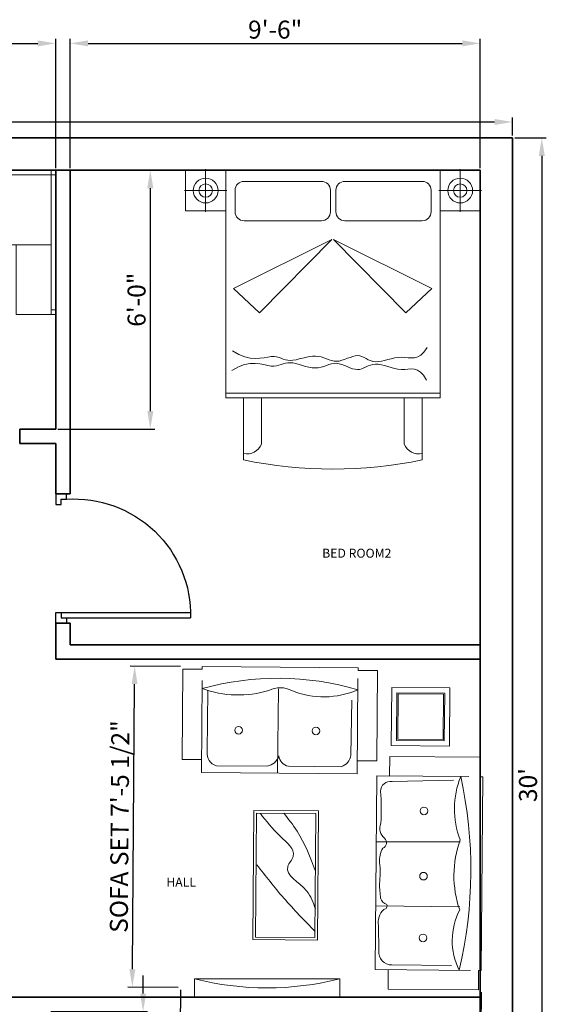
# Model space of a CAD drawing. Units: inches. Extents: x -24887 to 3061, y 1794 to 4919553.
# Tile 7 of 14: x 2328 to 2474, y 2076 to 2350. Entities that reach past the tile are written whole.
import ezdxf

# ---------------------------------------------------------------- set-up
doc = ezdxf.new("R2010")
doc.units = ezdxf.units.IN
for name, color, linetype, lineweight in [('A-ANNO-DIMS', 2, 'Continuous', 18), ('A-AREA-IDEN', 7, 'Continuous', 18), ('A-FURN', 8, 'Continuous', 18), ('door', 4, 'Continuous', 25), ('TV', 210, 'Continuous', 18), ('wall', 7, 'Continuous', 35)]:
    doc.layers.add(name, color=color, linetype=linetype, lineweight=lineweight)
doc.styles.get("Standard").update_dxf_attribs({"font": 'arial.ttf'})
doc.dimstyles.new('ISO-25', dxfattribs={"dimtxt": 5, "dimasz": 5, "dimexe": 1.25, "dimexo": 0.625, "dimtad": 1, "dimdec": 1, "dimlunit": 3, "dimtxsty": 'Standard', "dimcen": 2.5, "dimadec": 0, "dimazin": 0, "dimtfac": 1, "dimtdec": 1, "dimtmove": 0, "dimatfit": 3, "dimfxl": 1, "dimarcsym": 0})

# ---------------------------------------------------------------- blocks, each defined once
blk = doc.blocks.new('A$C4F543DC7')
for p, q in [((0.013, 3.35, -0.169), (3.313, 3.35, -0.169)), ((0.463, 3.35, -0.169), (0.013, 3.35, -0.169)), ((0.013, 2.896, -0.169), (0.013, 3.35, -0.169)), ((0.013, 3.35, -0.169), (0.013, 2.896, -0.169)), ((0.238, 3.123, -0.439), (0.238, 3.361, -0.439)), ((0.463, 3.35, -0.169), (0.463, 0.8, -0.169)), ((2.863, 3.35, -0.169), (0.463, 3.35, -0.169)), ((0.463, 2.896, -0.169), (0.463, 3.35, -0.169)), ((2.863, 0.8, -0.169), (2.863, 3.35, -0.169)), ((2.863, 3.35, -0.169), (3.313, 3.35, -0.169)), ((2.863, 2.896, -0.169), (2.863, 3.35, -0.169)), ((3.089, 3.123, -0.439), (3.089, 3.361, -0.439)), ((3.313, 3.35, -0.169), (3.313, 2.896, -0.169)), ((3.313, 3.35, -0.169), (3.313, 2.896, -0.169)), ((1.535, 3.226, -0.169), (0.668, 3.226, -0.169)), ((2.664, 3.226, -0.169), (1.797, 3.226, -0.169)), ((0.238, 3.123, -0.439), (0, 3.123, -0.439)), ((0.238, 3.123, -0.439), (0.476, 3.123, -0.439)), ((0.238, 3.123, -0.439), (0.238, 2.885, -0.439)), ((0.568, 3.126, -0.169), (0.568, 2.884, -0.169)), ((1.635, 2.884, -0.169), (1.635, 3.126, -0.169)), ((1.697, 3.126, -0.169), (1.697, 2.884, -0.169)), ((2.764, 2.884, -0.169), (2.764, 3.126, -0.169)), ((3.089, 3.123, -0.439), (2.851, 3.123, -0.439)), ((3.089, 3.123, -0.439), (3.089, 2.885, -0.439)), ((3.089, 3.123, -0.439), (3.327, 3.123, -0.439)), ((0.463, 2.896, -0.169), (0.013, 2.896, -0.169)), ((0.013, 2.896, -0.169), (0.463, 2.896, -0.169)), ((0.463, 0.8, -0.169), (0.463, 2.896, -0.169)), ((2.863, 2.896, -0.169), (2.863, 0.8, -0.169)), ((3.313, 2.896, -0.169), (2.863, 2.896, -0.169)), ((3.313, 2.896, -0.169), (2.863, 2.896, -0.169)), ((0.668, 2.784, -0.169), (1.535, 2.784, -0.169)), ((1.797, 2.784, -0.169), (2.664, 2.784, -0.169)), ((1.653, 2.573, -0.169), (0.55, 2.025, -0.169)), ((0.841, 1.752, -0.169), (1.653, 2.573, -0.169)), ((2.481, 1.752, -0.169), (1.669, 2.573, -0.169)), ((1.669, 2.573, -0.169), (2.772, 2.025, -0.169)), ((0.55, 2.025, -0.169), (0.841, 1.752, -0.169)), ((2.772, 2.025, -0.169), (2.481, 1.752, -0.169)), ((0.537, 1.327, -0.169), (0.609, 1.284, -0.169)), ((2.683, 1.312, -0.169), (2.718, 1.364, -0.169)), ((0.609, 1.284, -0.169), (0.676, 1.257, -0.169)), ((0.676, 1.257, -0.169), (0.737, 1.243, -0.169)), ((0.737, 1.243, -0.169), (0.794, 1.239, -0.169)), ((0.794, 1.239, -0.169), (0.846, 1.242, -0.169)), ((0.846, 1.242, -0.169), (0.893, 1.249, -0.169)), ((0.893, 1.249, -0.169), (0.935, 1.256, -0.169)), ((0.935, 1.256, -0.169), (0.972, 1.261, -0.169)), ((0.972, 1.261, -0.169), (1.004, 1.262, -0.169)), ((1.004, 1.262, -0.169), (1.033, 1.258, -0.169)), ((1.033, 1.258, -0.169), (1.06, 1.251, -0.169)), ((1.06, 1.251, -0.169), (1.084, 1.242, -0.169)), ((1.084, 1.242, -0.169), (1.108, 1.234, -0.169)), ((1.108, 1.234, -0.169), (1.132, 1.226, -0.169)), ((1.132, 1.226, -0.169), (1.158, 1.22, -0.169)), ((1.158, 1.22, -0.169), (1.185, 1.218, -0.169)), ((1.185, 1.218, -0.169), (1.216, 1.22, -0.169)), ((1.216, 1.22, -0.169), (1.25, 1.226, -0.169)), ((1.25, 1.226, -0.169), (1.285, 1.235, -0.169)), ((1.285, 1.235, -0.169), (1.322, 1.244, -0.169)), ((1.322, 1.244, -0.169), (1.359, 1.253, -0.169)), ((1.359, 1.253, -0.169), (1.396, 1.261, -0.169)), ((1.396, 1.261, -0.169), (1.433, 1.266, -0.169)), ((1.433, 1.266, -0.169), (1.468, 1.268, -0.169)), ((1.468, 1.268, -0.169), (1.501, 1.264, -0.169)), ((1.501, 1.264, -0.169), (1.532, 1.257, -0.169)), ((1.532, 1.257, -0.169), (1.562, 1.247, -0.169)), ((1.562, 1.247, -0.169), (1.591, 1.237, -0.169)), ((1.591, 1.237, -0.169), (1.62, 1.226, -0.169)), ((1.62, 1.226, -0.169), (1.648, 1.217, -0.169)), ((1.648, 1.217, -0.169), (1.676, 1.211, -0.169)), ((1.735, 1.212, -0.169), (1.765, 1.22, -0.169)), ((1.765, 1.22, -0.169), (1.795, 1.23, -0.169)), ((1.795, 1.23, -0.169), (1.826, 1.242, -0.169)), ((1.826, 1.242, -0.169), (1.856, 1.253, -0.169)), ((1.856, 1.253, -0.169), (1.885, 1.263, -0.169)), ((1.885, 1.263, -0.169), (1.913, 1.27, -0.169)), ((1.913, 1.27, -0.169), (1.94, 1.272, -0.169)), ((1.94, 1.272, -0.169), (1.965, 1.269, -0.169)), ((1.965, 1.269, -0.169), (1.989, 1.262, -0.169)), ((1.989, 1.262, -0.169), (2.012, 1.251, -0.169)), ((2.012, 1.251, -0.169), (2.036, 1.239, -0.169)), ((2.036, 1.239, -0.169), (2.06, 1.227, -0.169)), ((2.06, 1.227, -0.169), (2.085, 1.216, -0.169)), ((2.085, 1.216, -0.169), (2.112, 1.208, -0.169)), ((2.206, 1.21, -0.169), (2.242, 1.218, -0.169)), ((2.242, 1.218, -0.169), (2.279, 1.228, -0.169)), ((2.279, 1.228, -0.169), (2.317, 1.238, -0.169)), ((2.317, 1.238, -0.169), (2.356, 1.246, -0.169)), ((2.356, 1.246, -0.169), (2.394, 1.253, -0.169)), ((2.394, 1.253, -0.169), (2.433, 1.255, -0.169)), ((2.433, 1.255, -0.169), (2.47, 1.253, -0.169)), ((2.47, 1.253, -0.169), (2.506, 1.249, -0.169)), ((2.506, 1.249, -0.169), (2.542, 1.246, -0.169)), ((2.542, 1.246, -0.169), (2.578, 1.248, -0.169)), ((2.578, 1.248, -0.169), (2.613, 1.257, -0.169)), ((2.613, 1.257, -0.169), (2.648, 1.277, -0.169)), ((2.648, 1.277, -0.169), (2.683, 1.312, -0.169)), ((0.533, 1.105, -0.169), (0.607, 1.146, -0.169)), ((0.607, 1.146, -0.169), (0.674, 1.171, -0.169)), ((0.674, 1.171, -0.169), (0.736, 1.183, -0.169)), ((0.736, 1.183, -0.169), (0.793, 1.185, -0.169)), ((0.793, 1.185, -0.169), (0.845, 1.18, -0.169)), ((0.845, 1.18, -0.169), (0.891, 1.172, -0.169)), ((0.891, 1.172, -0.169), (0.933, 1.163, -0.169)), ((0.933, 1.163, -0.169), (0.97, 1.156, -0.169)), ((0.97, 1.156, -0.169), (1.003, 1.155, -0.169)), ((1.003, 1.155, -0.169), (1.032, 1.158, -0.169)), ((1.032, 1.158, -0.169), (1.058, 1.164, -0.169)), ((1.058, 1.164, -0.169), (1.083, 1.172, -0.169)), ((1.083, 1.172, -0.169), (1.107, 1.18, -0.169)), ((1.107, 1.18, -0.169), (1.132, 1.187, -0.169)), ((1.132, 1.187, -0.169), (1.157, 1.192, -0.169)), ((1.157, 1.192, -0.169), (1.185, 1.193, -0.169)), ((1.185, 1.193, -0.169), (1.216, 1.19, -0.169)), ((1.216, 1.19, -0.169), (1.249, 1.183, -0.169)), ((1.249, 1.183, -0.169), (1.284, 1.173, -0.169)), ((1.284, 1.173, -0.169), (1.321, 1.163, -0.169)), ((1.321, 1.163, -0.169), (1.358, 1.152, -0.169)), ((1.358, 1.152, -0.169), (1.394, 1.143, -0.169)), ((1.394, 1.143, -0.169), (1.431, 1.137, -0.169)), ((1.431, 1.137, -0.169), (1.466, 1.135, -0.169)), ((1.466, 1.135, -0.169), (1.499, 1.137, -0.169)), ((1.499, 1.137, -0.169), (1.531, 1.143, -0.169)), ((1.531, 1.143, -0.169), (1.561, 1.152, -0.169)), ((1.561, 1.152, -0.169), (1.59, 1.162, -0.169)), ((1.59, 1.162, -0.169), (1.619, 1.172, -0.169)), ((1.619, 1.172, -0.169), (1.648, 1.18, -0.169)), ((1.648, 1.18, -0.169), (1.676, 1.185, -0.169)), ((1.676, 1.211, -0.169), (1.705, 1.209, -0.169)), ((1.676, 1.185, -0.169), (1.705, 1.186, -0.169)), ((1.705, 1.209, -0.169), (1.735, 1.212, -0.169)), ((1.705, 1.186, -0.169), (1.734, 1.182, -0.169)), ((1.734, 1.182, -0.169), (1.764, 1.173, -0.169)), ((1.764, 1.173, -0.169), (1.794, 1.162, -0.169)), ((1.794, 1.162, -0.169), (1.824, 1.149, -0.169)), ((1.824, 1.149, -0.169), (1.854, 1.137, -0.169)), ((1.854, 1.137, -0.169), (1.883, 1.126, -0.169)), ((1.883, 1.126, -0.169), (1.911, 1.119, -0.169)), ((1.911, 1.119, -0.169), (1.937, 1.115, -0.169)), ((1.937, 1.115, -0.169), (1.963, 1.118, -0.169)), ((1.963, 1.118, -0.169), (1.987, 1.124, -0.169)), ((1.987, 1.124, -0.169), (2.011, 1.134, -0.169)), ((2.011, 1.134, -0.169), (2.034, 1.145, -0.169)), ((2.034, 1.145, -0.169), (2.059, 1.157, -0.169)), ((2.059, 1.157, -0.169), (2.084, 1.167, -0.169)), ((2.084, 1.167, -0.169), (2.111, 1.174, -0.169)), ((2.111, 1.174, -0.169), (2.14, 1.177, -0.169)), ((2.112, 1.208, -0.169), (2.141, 1.204, -0.169)), ((2.14, 1.177, -0.169), (2.172, 1.175, -0.169)), ((2.141, 1.204, -0.169), (2.172, 1.205, -0.169)), ((2.172, 1.205, -0.169), (2.206, 1.21, -0.169)), ((2.172, 1.175, -0.169), (2.206, 1.169, -0.169)), ((2.206, 1.169, -0.169), (2.241, 1.16, -0.169)), ((2.241, 1.16, -0.169), (2.278, 1.149, -0.169)), ((2.278, 1.149, -0.169), (2.316, 1.138, -0.169)), ((2.316, 1.138, -0.169), (2.354, 1.128, -0.169)), ((2.354, 1.128, -0.169), (2.392, 1.121, -0.169)), ((2.392, 1.121, -0.169), (2.43, 1.117, -0.169)), ((2.43, 1.117, -0.169), (2.468, 1.118, -0.169)), ((2.468, 1.118, -0.169), (2.504, 1.121, -0.169)), ((2.504, 1.121, -0.169), (2.54, 1.123, -0.169)), ((2.54, 1.123, -0.169), (2.576, 1.12, -0.169)), ((2.576, 1.12, -0.169), (2.611, 1.109, -0.169)), ((2.611, 1.109, -0.169), (2.645, 1.088, -0.169)), ((2.645, 1.088, -0.169), (2.679, 1.052, -0.169)), ((2.679, 1.052, -0.169), (2.712, 0.999, -0.169)), ((0.463, 0.85, -0.169), (2.863, 0.85, -0.169)), ((0.463, 0.8, -0.169), (2.863, 0.8, -0.169)), ((0.663, 0.8, -0.169), (0.463, 0.8, -0.169)), ((0.663, 0.8, -0.169), (2.663, 0.8, -0.169)), ((0.663, 0.104, -0.169), (0.663, 0.8, -0.169)), ((0.663, 0.104, -0.169), (0.663, 0.8, -0.169)), ((0.863, 0.281, -0.169), (0.863, 0.8, -0.169)), ((2.463, 0.8, -0.169), (2.463, 0.281, -0.169)), ((2.863, 0.8, -0.169), (2.663, 0.8, -0.169)), ((2.663, 0.8, -0.169), (2.663, 0.104, -0.169)), ((2.663, 0.8, -0.169), (2.663, 0.104, -0.169))]:
    blk.add_line(p, q)
for centre, radius in [((0.238, 3.123, -0.439), 0.139), ((3.089, 3.123, -0.439), 0.139), ((0.238, 3.123, -0.439), 0.075), ((3.089, 3.123, -0.439), 0.075)]:
    blk.add_circle(centre, radius)
for centre, radius, start, end in [((0.668, 3.126, -0.169), 0.1, 90, 180), ((1.535, 3.126, -0.169), 0.1, 0, 90), ((1.797, 3.126, -0.169), 0.1, 90, 180), ((2.664, 3.126, -0.169), 0.1, 0, 90), ((0.668, 2.884, -0.169), 0.1, 180, 270), ((1.535, 2.884, -0.169), 0.1, 270, 0), ((1.797, 2.884, -0.169), 0.1, 180, 270), ((2.664, 2.884, -0.169), 0.1, 270, 0), ((0.699, 0.347, -0.169), 0.177, 258.2616, 338.032), ((2.627, 0.347, -0.169), 0.177, 201.968, 281.7384), ((1.663, 4.86, -0.169), 4.86, 258.1252, 281.8748), ((1.663, 4.86, -0.169), 4.86, 258.1252, 281.8748)]:
    blk.add_arc(centre, radius, start, end)
blk = doc.blocks.new('A$C412119AE')
for p, q in [((1765.9, 2176), (1765.9, 2326)), ((1765.9, 2326), (2465.9, 2326)), ((2465.9, 2326), (2465.9, 2176)), ((1665.9, 2176), (1765.9, 2176)), ((1665.9, 2176), (1665.9, 970.8)), ((2379.1, 2176), (1665.9, 2176)), ((2465.9, 2176), (2485.9, 2176)), ((2485.9, 2176), (2485.9, 970.8)), ((1719.4, 1668.1), (1719.4, 2061.3)), ((1825.7, 2132.2), (2302.7, 2132.2)), ((1375.4, 1768.9), (375.4, 1768.9)), ((375.4, 1768.9), (375.4, 1268.9)), ((1375.4, 1268.9), (1375.4, 1768.9)), ((1355.4, 1748.9), (395.4, 1748.9)), ((395.4, 1748.9), (395.4, 1288.9)), ((1355.4, 1288.9), (1355.4, 1748.9)), ((1669.2, 1587.6), (2319.2, 1585.7)), ((1719.4, 1094.5), (1719.4, 1503.8)), ((375.4, 1268.9), (1375.4, 1268.9)), ((395.4, 1288.9), (1355.4, 1288.9)), ((2235, 1017.2), (1809.6, 1020.4)), ((1665.9, 970.8), (2404.3, 970.8)), ((1765.9, 820.8), (1765.9, 970.8)), ((2485.9, 970.8), (2465.9, 970.8)), ((2465.9, 970.8), (2465.9, 820.8)), ((150, 820), (150, 81.6)), ((1650, 820), (150, 820)), ((490.8, 797.2), (296.7, 793)), ((642.7, 820), (640.8, 170)), ((1139.6, 820), (1143.5, 170)), ((1650, 106.9), (1650, 820)), ((1650, 820), (1650, 720)), ((2465.9, 820.8), (1765.9, 820.8)), ((0, 20), (0, 720)), ((0, 720), (150, 720)), ((187.2, 692), (187.2, 228.9)), ((1620.5, 224.7), (1607.9, 700.4)), ((1650, 720), (1800, 720)), ((1800, 720), (1800, 20)), ((1885.8, 708.9), (1885.8, 258.9)), ((2335.8, 708.9), (1885.8, 708.9)), ((2335.8, 258.9), (2335.8, 708.9)), ((1925.8, 668.9), (1925.8, 298.9)), ((2295.8, 668.9), (1925.8, 668.9)), ((1935.8, 658.9), (1935.8, 308.9)), ((2285.8, 658.9), (1935.8, 658.9)), ((2285.8, 308.9), (2285.8, 658.9)), ((2295.8, 298.9), (2295.8, 668.9)), ((1935.8, 308.9), (2285.8, 308.9)), ((1885.8, 258.9), (2335.8, 258.9)), ((1925.8, 298.9), (2295.8, 298.9)), ((150, 20), (0, 20)), ((150, 0), (150, 20)), ((1650, 20), (1650, 0)), ((1800, 20), (1650, 20)), ((1650, 0), (150, 0))]:
    blk.add_line(p, q)
for centre in [(1995.2, 1891.7), (1995.2, 1293.1), (398.2, 452), (876.5, 452), (1381.8, 452)]:
    blk.add_circle(centre, 29.5)
for centre, radius, start, end in [((3089.3, 1902.2), 820.4, 160.50304, 197.27883), ((202.9, 1573.4), 2197.3, 344.08302, 15.91698), ((1812.8, 2036.4), 96.7, 82.30019, 165.08006), ((1830, 1685.8), 112, 189.0797, 254.44081), ((2133.5, 1569.9), 193.8, 332.79347, 27.20653), ((1809.1, 1487.1), 91.2, 95.74421, 169.48399), ((2917.4, 1237.9), 658.1, 158.30056, 203.94833), ((1824.2, 1130.1), 110.7, 198.77187, 262.42669), ((284.9, 696), 97.7, 83.05444, 182.36446), ((516, 656.3), 143.2, 45.31905, 100.10139), ((721.1, 716.6), 67.9, 104.67166, 165.32844), ((1108.9, -2844), 3648.9, 94.62092, 96.37281), ((897.6, 1374.7), 587.5, 261.9179, 278.0821), ((996.1, 612.3), 181.4, 58.97104, 95.03964), ((1133, 788.8), 48.2, 205.88938, 315.66926), ((1244.1, 695.8), 96.9, 66.28266, 142.29634), ((1373.1, 2811.3), 2028.7, 267.45837, 274.48249), ((1532.5, 712.5), 76.3, 350.88786, 90.69758), ((643.8, 758.5), 27.2, 180.80594, 295.18319), ((383.4, -290.5), 516.3, 63.11882, 116.88118), ((900, 3466.4), 3380.7, 257.18237, 282.81763), ((888.2, -595.2), 811.8, 70.47891, 109.52109), ((1404.7, -453), 669.5, 68.50957, 111.49043)]:
    blk.add_arc(centre, radius, start, end)
for points, knots in [([(954.7, 1741.3), (867.9, 1672.9), (688.2, 1531.3), (525.8, 1370), (441.9, 1286.7)], [0, 0, 0, 0, 331.319965, 685.817203, 685.817203, 685.817203, 685.817203]), ([(1351, 1718), (1294.3, 1672.1), (1194, 1591.1), (1053.5, 1416.2), (895.9, 1563.2), (786.6, 1342.9), (665.1, 1302.7), (616.7, 1286.7)], [0, 0, 0, 0, 235.219039, 416.259432, 507.480442, 744.13898, 900.517858, 900.517858, 900.517858, 900.517858]), ([(1356.8, 1537.3), (1311.3, 1500.6), (1176.6, 1392.3), (1015, 1328.7), (908.1, 1286.7)], [0, 0, 0, 0, 174.836893, 516.353531, 516.353531, 516.353531, 516.353531])]:
    blk.add_open_spline(points, degree=3, knots=knots)
blk = doc.blocks.new('*D30')
at = {"layer": 'A-ANNO-DIMS', "color": 0, "lineweight": -2, "transparency": 16777216}
for p, q in [((2164.92, 2317.57), (2164.92, 2322.63)), ((2464.92, 2317.57), (2464.92, 2322.63)), ((2169.92, 2321.38), (2459.92, 2321.38))]:
    blk.add_line(p, q, dxfattribs=at)
at = {"layer": 'A-ANNO-DIMS', "color": 0, "transparency": 16777216}
for points in [[(2169.92, 2322.21), (2169.92, 2320.55), (2164.92, 2321.38)], [(2459.92, 2322.21), (2459.92, 2320.55), (2464.92, 2321.38)]]:
    blk.add_solid(points, dxfattribs=at)
at = {"layer": 'Defpoints', "color": 0, "transparency": 16777216}
for p in [(2464.92, 2321.38), (2164.92, 2316.94), (2464.92, 2316.94)]:
    blk.add_point(p, dxfattribs=at)
at = {"layer": 'A-ANNO-DIMS', "color": 0, "transparency": 16777216, "insert": (2314.92, 2324.56), "char_height": 5, "attachment_point": 5}
blk.add_mtext("25'", dxfattribs=at)
blk = doc.blocks.new('*D31')
at = {"layer": 'A-ANNO-DIMS', "color": 0, "lineweight": -2, "transparency": 16777216}
for p, q in [((2465.55, 2316.94), (2474.28, 2316.94)), ((2473.03, 2311.94), (2473.03, 1961.94)), ((2465.55, 1956.94), (2474.28, 1956.94))]:
    blk.add_line(p, q, dxfattribs=at)
at = {"layer": 'A-ANNO-DIMS', "color": 0, "transparency": 16777216}
for points in [[(2472.2, 2311.94), (2473.87, 2311.94), (2473.03, 2316.94)], [(2472.2, 1961.94), (2473.87, 1961.94), (2473.03, 1956.94)]]:
    blk.add_solid(points, dxfattribs=at)
at = {"layer": 'Defpoints', "color": 0, "transparency": 16777216}
for p in [(2464.92, 2316.94), (2464.92, 1956.94), (2473.03, 1956.94)]:
    blk.add_point(p, dxfattribs=at)
at = {"layer": 'A-ANNO-DIMS', "color": 0, "transparency": 16777216, "insert": (2469.85, 2136.94), "char_height": 5, "attachment_point": 5, "rotation": 90}
blk.add_mtext("30'", dxfattribs=at)
blk = doc.blocks.new('DOOR-SINGLE-36IN')
for p, q in [((34.5, 36), (37.5, 36)), ((34.5, 34.5), (34.5, 36)), ((37.5, 36), (37.5, 33)), ((36, 34.5), (34.5, 34.5)), ((36, 33), (36, 34.5)), ((37.5, 33), (36, 33)), ((36, 3), (0, 3)), ((37.5, 3), (36, 3)), ((36, 3), (36, 1.5)), ((37.5, 0), (37.5, 3)), ((36, 1.5), (0, 1.5)), ((36, 1.5), (34.5, 1.5)), ((34.5, 1.5), (34.5, 0)), ((34.5, 0), (37.5, 0))]:
    blk.add_line(p, q)
blk.add_arc((32.32, 2.25), 32.32, 86.1244, 181.3295)
blk = doc.blocks.new('DESK-CORNER-WITH-CHAIR')
for p, q in [((0, 40.37), (40.11, 40.37)), ((0, 19.67), (0, 40.37)), ((0, 39.07), (40.11, 39.07)), ((1.29, 39.07), (1.29, 40.37)), ((38.82, 40.37), (38.82, 19.67)), ((40.11, 40.37), (40.11, 0.26)), ((38.82, 19.67), (0, 19.67)), ((29.11, 19.67), (38.82, 19.67)), ((29.11, 0.26), (29.11, 19.67)), ((38.82, 19.67), (38.82, 0.26)), ((7.89, 10.98), (7.93, 2.72)), ((8.97, 10.98), (9.02, 1.91)), ((9.17, 10.98), (9.17, 11.46)), ((9.17, 10.99), (9.18, 9.53)), ((10.75, 13.07), (10.91, 13.07)), ((11.62, 13.07), (10.91, 13.07)), ((17.49, 13.1), (18.37, 13.11)), ((19.98, 11.02), (19.97, 11.52)), ((19.98, 11.02), (19.98, 9.56)), ((20.18, 11.01), (20.22, 1.94)), ((21.26, 11.02), (21.3, 2.76)), ((9.17, 9.52), (9.22, 2.03)), ((19.99, 9.54), (20.03, 2.06)), ((40.11, 0.26), (29.11, 0.26)), ((40.11, 1.55), (38.82, 1.55))]:
    blk.add_line(p, q)
for centre, radius, start, end in [((8.43, 10.73), 0.593, 24.5958, 155.829), ((10.76, 11.47), 1.6, 90.3083, 180.3083), ((14.78, -28.11), 41.3, 86.2317, 94.3849), ((18.38, 11.51), 1.6, 0.3083, 90.3083), ((20.72, 10.77), 0.593, 24.7876, 156.0208), ((20.52, 10.77), 0.593, 204.3355, 206.5711), ((9.82, 2.64), 3.42, 74.7531, 100.4859), ((14.4, 34.16), 28.46, 262.2773, 278.3393), ((19.33, 2.69), 3.42, 78.6001, 104.4332), ((10.57, 1.77), 1.37, 80.5561, 260.4095), ((9.82, 2.64), 2.42, 74.7531, 104.4332), ((10.9, 5.33), 2.21, 220.0354, 267.4848), ((9.82, 1.7), 2.42, 74.7531, 104.4332), ((14.4, 34.16), 29.46, 262.2773, 278.3393), ((14.4, 33.22), 29.46, 262.2773, 278.3393), ((14.95, 25.37), 22.63, 259.4369, 269.1516), ((14.03, 25.37), 22.63, 271.465, 281.1797), ((18.3, 5.37), 2.21, 273.1318, 320.9947), ((18.66, 1.82), 1.37, 280.2071, 100.0605), ((19.33, 2.69), 2.42, 73.6429, 104.4332), ((19.33, 1.75), 2.42, 73.6429, 104.4332), ((20.48, 2.72), 0.821, 251.7835, 2.9643), ((8.75, 2.68), 0.821, 177.6524, 288.8331), ((14.52, 20.73), 20.73, 258.3982, 282.2184)]:
    blk.add_arc(centre, radius, start, end)
blk = doc.blocks.new('*D52')
at = {"layer": 'A-ANNO-DIMS', "color": 0, "lineweight": -2, "transparency": 16777216}
for p, q in [((2311.01, 2162.63), (2321.67, 2162.63)), ((2320.42, 2100.73), (2320.42, 2157.63)), ((2311.01, 2095.73), (2321.67, 2095.73))]:
    blk.add_line(p, q, dxfattribs=at)
at = {"layer": 'A-ANNO-DIMS', "color": 0, "transparency": 16777216}
for points in [[(2319.59, 2157.63), (2321.25, 2157.63), (2320.42, 2162.63)], [(2319.59, 2100.73), (2321.25, 2100.73), (2320.42, 2095.73)]]:
    blk.add_solid(points, dxfattribs=at)
at = {"layer": 'Defpoints', "color": 0, "transparency": 16777216}
for p in [(2310.39, 2162.63), (2320.42, 2162.63), (2310.39, 2095.73)]:
    blk.add_point(p, dxfattribs=at)
at = {"layer": 'A-ANNO-DIMS', "color": 0, "transparency": 16777216, "insert": (2317.21, 2129.18), "char_height": 5, "attachment_point": 5, "rotation": 90}
blk.add_mtext('DINING SET 5\'-7"', dxfattribs=at)
blk = doc.blocks.new('*D60')
at = {"layer": 'A-ANNO-DIMS', "color": 0, "lineweight": -2, "transparency": 16777216}
for p, q in [((2372.65, 2169.91), (2358.63, 2170.02)), ((2359.25, 2085.71), (2359.85, 2165.01)), ((2371.98, 2080.61), (2357.96, 2080.72))]:
    blk.add_line(p, q, dxfattribs=at)
at = {"layer": 'A-ANNO-DIMS', "color": 0, "transparency": 16777216}
for points in [[(2359.01, 2165.01), (2360.68, 2165), (2359.88, 2170.01)], [(2358.41, 2085.72), (2360.08, 2085.7), (2359.21, 2080.71)]]:
    blk.add_solid(points, dxfattribs=at)
at = {"layer": 'Defpoints', "color": 0, "transparency": 16777216}
for p in [(2359.88, 2170.01), (2373.28, 2169.91), (2372.6, 2080.61)]:
    blk.add_point(p, dxfattribs=at)
at = {"layer": 'A-ANNO-DIMS', "color": 0, "transparency": 16777216, "insert": (2356.33, 2125.38), "char_height": 5, "attachment_point": 5, "rotation": 89.5659}
blk.add_mtext('SOFA SET 7\'-5 1/2"', dxfattribs=at)
blk = doc.blocks.new('*D61')
at = {"layer": 'A-ANNO-DIMS', "color": 0, "lineweight": -2, "transparency": 16777216}
for p, q in [((2372.6, 2079.98), (2372.49, 2065.97)), ((2456.15, 2079.35), (2456.04, 2065.33)), ((2451.05, 2066.62), (2377.5, 2067.18))]:
    blk.add_line(p, q, dxfattribs=at)
at = {"layer": 'A-ANNO-DIMS', "color": 0, "transparency": 16777216}
for points in [[(2377.51, 2068.01), (2377.49, 2066.34), (2372.5, 2067.22)], [(2451.06, 2067.45), (2451.04, 2065.79), (2456.05, 2066.58)]]:
    blk.add_solid(points, dxfattribs=at)
at = {"layer": 'Defpoints', "color": 0, "transparency": 16777216}
for p in [(2372.6, 2080.61), (2456.15, 2079.98), (2372.5, 2067.22)]:
    blk.add_point(p, dxfattribs=at)
at = {"layer": 'A-ANNO-DIMS', "color": 0, "transparency": 16777216, "insert": (2414.3, 2070.11), "char_height": 5, "attachment_point": 5, "rotation": 359.5659}
blk.add_mtext('6\'-11 1/2"', dxfattribs=at)
blk = doc.blocks.new('*D84')
at = {"layer": 'A-ANNO-DIMS', "color": 0, "lineweight": -2, "transparency": 16777216}
for p, q in [((2297.92, 2308.57), (2297.92, 2344.49)), ((2337.92, 2308.57), (2337.92, 2344.49)), ((2302.92, 2343.24), (2332.92, 2343.24))]:
    blk.add_line(p, q, dxfattribs=at)
at = {"layer": 'A-ANNO-DIMS', "color": 0, "transparency": 16777216}
for points in [[(2302.92, 2344.07), (2302.92, 2342.41), (2297.92, 2343.24)], [(2332.92, 2344.07), (2332.92, 2342.41), (2337.92, 2343.24)]]:
    blk.add_solid(points, dxfattribs=at)
at = {"layer": 'Defpoints', "color": 0, "transparency": 16777216}
for p in [(2337.92, 2343.24), (2297.92, 2307.94), (2337.92, 2307.94)]:
    blk.add_point(p, dxfattribs=at)
at = {"layer": 'A-ANNO-DIMS', "color": 0, "transparency": 16777216, "insert": (2317.92, 2346.42), "char_height": 5, "attachment_point": 5}
blk.add_mtext('3\'-4"', dxfattribs=at)
blk = doc.blocks.new('*D85')
at = {"layer": 'A-ANNO-DIMS', "color": 0, "lineweight": -2, "transparency": 16777216}
for p, q in [((2341.92, 2308.57), (2341.92, 2344.49)), ((2455.92, 2308.57), (2455.92, 2344.49)), ((2346.92, 2343.24), (2450.92, 2343.24))]:
    blk.add_line(p, q, dxfattribs=at)
at = {"layer": 'A-ANNO-DIMS', "color": 0, "transparency": 16777216}
for points in [[(2346.92, 2344.07), (2346.92, 2342.41), (2341.92, 2343.24)], [(2450.92, 2344.07), (2450.92, 2342.41), (2455.92, 2343.24)]]:
    blk.add_solid(points, dxfattribs=at)
at = {"layer": 'Defpoints', "color": 0, "transparency": 16777216}
for p in [(2455.92, 2343.24), (2341.92, 2307.94), (2455.92, 2307.94)]:
    blk.add_point(p, dxfattribs=at)
at = {"layer": 'A-ANNO-DIMS', "color": 0, "transparency": 16777216, "insert": (2398.92, 2346.42), "char_height": 5, "attachment_point": 5}
blk.add_mtext('9\'-6"', dxfattribs=at)
blk = doc.blocks.new('*D92')
at = {"layer": 'A-ANNO-DIMS', "color": 0, "lineweight": -2, "transparency": 16777216}
for p, q in [((2338.55, 2307.94), (2365.47, 2307.94)), ((2364.22, 2302.94), (2364.22, 2240.94)), ((2338.55, 2235.94), (2365.47, 2235.94))]:
    blk.add_line(p, q, dxfattribs=at)
at = {"layer": 'A-ANNO-DIMS', "color": 0, "transparency": 16777216}
for points in [[(2363.39, 2302.94), (2365.06, 2302.94), (2364.22, 2307.94)], [(2363.39, 2240.94), (2365.06, 2240.94), (2364.22, 2235.94)]]:
    blk.add_solid(points, dxfattribs=at)
at = {"layer": 'Defpoints', "color": 0, "transparency": 16777216}
for p in [(2337.92, 2307.94), (2337.92, 2235.94), (2364.22, 2235.94)]:
    blk.add_point(p, dxfattribs=at)
at = {"layer": 'A-ANNO-DIMS', "color": 0, "transparency": 16777216, "insert": (2361.05, 2271.94), "char_height": 5, "attachment_point": 5, "rotation": 90}
blk.add_mtext('6\'-0"', dxfattribs=at)
blk = doc.blocks.new('*D98')
at = {"layer": 'A-ANNO-DIMS', "color": 0, "lineweight": -2, "transparency": 16777216}
for p, q in [((2362.22, 2078.94), (2362.22, 2083.94)), ((2336.55, 2073.94), (2363.47, 2073.94)), ((2362.22, 2073.94), (2362.22, 2067.94)), ((2336.55, 2067.94), (2363.47, 2067.94)), ((2362.22, 2062.94), (2362.22, 2043.4))]:
    blk.add_line(p, q, dxfattribs=at)
at = {"layer": 'A-ANNO-DIMS', "color": 0, "transparency": 16777216}
for points in [[(2361.39, 2078.94), (2363.06, 2078.94), (2362.22, 2073.94)], [(2361.39, 2062.94), (2363.06, 2062.94), (2362.22, 2067.94)]]:
    blk.add_solid(points, dxfattribs=at)
at = {"layer": 'Defpoints', "color": 0, "transparency": 16777216}
for p in [(2335.92, 2073.94), (2335.92, 2067.94), (2362.22, 2067.94)]:
    blk.add_point(p, dxfattribs=at)
at = {"layer": 'A-ANNO-DIMS', "color": 0, "transparency": 16777216, "insert": (2359.05, 2050.67), "char_height": 5, "attachment_point": 5, "rotation": 90}
blk.add_mtext('0\'-6"', dxfattribs=at)

msp = doc.modelspace()

# ---------------------------------------------------------------- linework, layer by layer
at = {"layer": 'TV'}
msp.add_lwpolyline([(2376.49, 2077.94), (2416.86, 2077.94), (2416.86, 2083.04), (2376.49, 2083.04)], close=True, dxfattribs=at)
msp.add_arc((2396.68, 2161.63), 81.14, 255.5981, 284.4019, dxfattribs=at)
at = {"layer": 'wall'}
for p, q in [((2464.92, 2316.94), (2164.92, 2316.94)), ((2464.92, 1956.94), (2464.92, 2316.94)), ((2455.92, 2307.94), (2173.92, 2307.94)), ((2337.92, 2307.94), (2337.92, 2235.94)), ((2341.92, 2307.94), (2341.92, 2217.94)), ((2455.92, 1965.94), (2455.92, 2307.94)), ((2337.92, 2235.94), (2327.92, 2235.94)), ((2327.92, 2235.94), (2327.92, 2231.94)), ((2337.92, 2231.94), (2327.92, 2231.94)), ((2337.92, 2231.94), (2337.92, 2217.94)), ((2341.92, 2217.94), (2337.92, 2217.94)), ((2341.92, 2181.94), (2337.92, 2181.94)), ((2337.92, 2181.94), (2337.92, 2171.94)), ((2341.92, 2181.94), (2341.92, 2175.94)), ((2455.92, 2175.94), (2341.92, 2175.94)), ((2455.92, 2171.94), (2337.92, 2171.94)), ((2455.92, 2077.94), (2225.92, 2077.94))]:
    msp.add_line(p, q, dxfattribs=at)

# ---------------------------------------------------------------- block references
at = {"layer": 'A-FURN'}
msp.add_blockref('DESK-CORNER-WITH-CHAIR', (2297.81, 2267.57), dxfattribs=at)
at = {"layer": 'A-FURN', "xscale": 24.81469674658305, "yscale": 24.81469674658305, "zscale": 24.81469674658305}
msp.add_blockref('A$C4F543DC7', (2373.7, 2224.81, 4.19), dxfattribs=at)
at = {"layer": 'A-FURN', "xscale": 0.0359212862277956, "yscale": 0.0359212862277956, "zscale": 0.0359212862277956, "rotation": 89.56594542985536}
msp.add_blockref('A$C412119AE', (2456.15, 2079.98), dxfattribs=at)
at = {"layer": 'door', "extrusion": (0, 0, -1), "zscale": -1}
msp.add_blockref('DOOR-SINGLE-36IN', (-2375.42, 2181.94), dxfattribs=at)

# ---------------------------------------------------------------- texts
at = {"layer": 'A-AREA-IDEN', "char_height": 2.5, "attachment_point": 1}
for s, insert in [('BED ROOM2', (2411.99, 2202.67)), ('HALL', (2368.67, 2111.16))]:
    msp.add_mtext_dynamic_manual_height_columns(s, width=34.2323, gutter_width=12.5, heights=[0], dxfattribs=dict(at, insert=insert))

# ---------------------------------------------------------------- dimensions: what is measured, and where the dimension line sits
at = {"layer": 'A-ANNO-DIMS'}
for base, p1, p2, override, picture, middle in [((2337.92, 2343.24), (2297.92, 2307.94), (2337.92, 2307.94), {"dimdec": 1, "dimlfac": 1, "dimrnd": 0, "dimzin": 1, "dimdsep": 46, "dimlunit": 4, "dimfrac": 2}, '*D84', (2317.92, 2346.42)), ((2455.92, 2343.24), (2341.92, 2307.94), (2455.92, 2307.94), {"dimdec": 1, "dimlfac": 1, "dimrnd": 0, "dimzin": 1, "dimdsep": 46, "dimlunit": 4, "dimfrac": 2}, '*D85', (2398.92, 2346.42)), ((2464.92, 2321.38), (2164.92, 2316.94), (2464.92, 2316.94), {"dimclrd": 0, "dimclre": 0, "dimclrt": 0}, '*D30', (2314.92, 2324.56))]:
    dim = msp.add_linear_dim(base=base, p1=p1, p2=p2, dimstyle='ISO-25', override=override, dxfattribs=at)
    dim.commit()
    dim.dimension.update_dxf_attribs({"geometry": picture, "text_midpoint": middle})
for base, p1, p2, angle, override, picture, middle in [((2473.03, 1956.94), (2464.92, 2316.94), (2464.92, 1956.94), 90, {"dimclrd": 0, "dimclre": 0, "dimclrt": 0}, '*D31', (2469.85, 2136.94)), ((2364.22, 2235.94), (2337.92, 2307.94), (2337.92, 2235.94), 270, {"dimdec": 1, "dimlfac": 1, "dimrnd": 0, "dimzin": 1, "dimdsep": 46, "dimlunit": 4, "dimfrac": 2}, '*D92', (2361.05, 2271.94)), ((2362.22, 2067.94), (2335.92, 2073.94), (2335.92, 2067.94), 270, {"dimdec": 1, "dimlfac": 1, "dimrnd": 0, "dimzin": 1, "dimdsep": 46, "dimlunit": 4, "dimfrac": 2}, '*D98', (2359.05, 2050.67)), ((2372.5, 2067.22), (2456.15, 2079.98), (2372.6, 2080.61), 179.5659, {"dimdec": 1, "dimlfac": 1, "dimrnd": 0, "dimzin": 1, "dimdsep": 46, "dimlunit": 4, "dimfrac": 2}, '*D61', (2414.3, 2070.11))]:
    dim = msp.add_linear_dim(base=base, p1=p1, p2=p2, angle=angle, dimstyle='ISO-25', override=override, dxfattribs=at)
    dim.commit()
    dim.dimension.update_dxf_attribs({"geometry": picture, "text_midpoint": middle})
for base, p1, p2, angle, text, picture, middle in [((2359.88, 2170.01), (2372.6, 2080.61), (2373.28, 2169.91), 89.5659, 'SOFA SET <>', '*D60', (2356.33, 2125.38)), ((2320.42, 2162.63), (2310.39, 2095.73), (2310.39, 2162.63), 90, 'DINING SET <>', '*D52', (2317.21, 2129.18))]:
    dim = msp.add_linear_dim(base=base, p1=p1, p2=p2, angle=angle, text=text, dimstyle='ISO-25', override={"dimdec": 1, "dimlfac": 1, "dimrnd": 0, "dimzin": 1, "dimdsep": 46, "dimlunit": 4, "dimfrac": 2}, dxfattribs=at)
    dim.commit()
    dim.dimension.update_dxf_attribs({"geometry": picture, "text_midpoint": middle})

doc.saveas('drawing.dxf')
